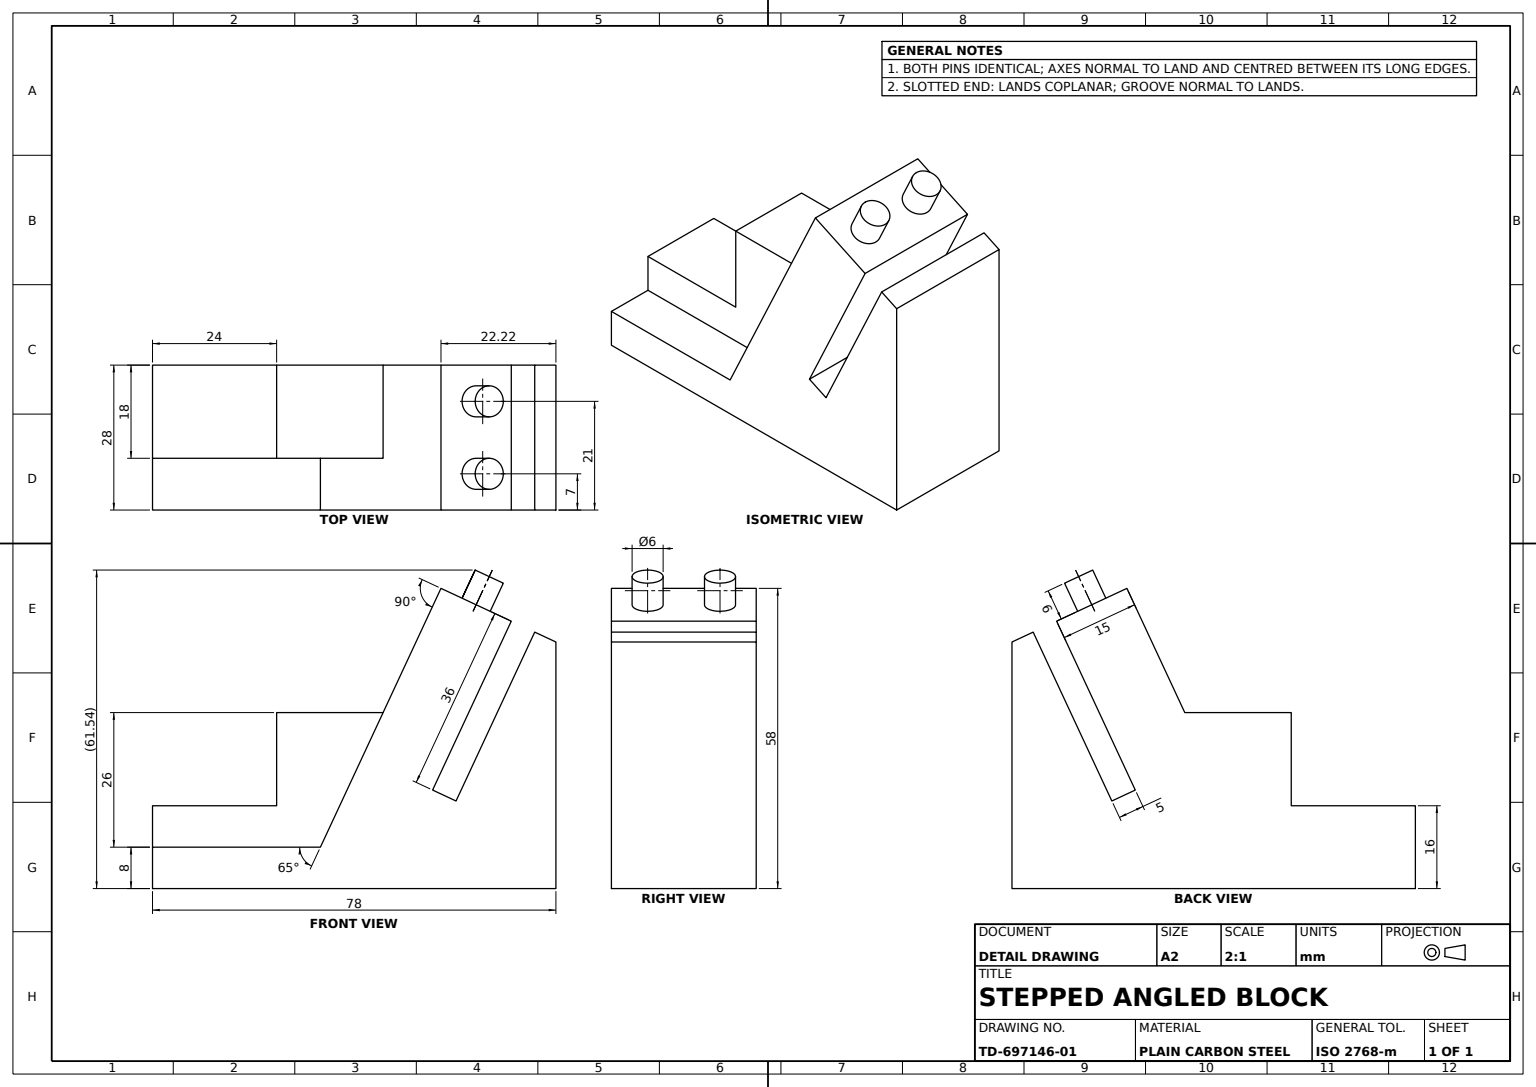
from build123d import *

# Parameters (mm, degrees)
STEPPED_BASE_BLOCK_DEPTH = 28
RISER_BLOCK_16X18_REACH  = 103.153
RISER_BLOCK_SKETCH_W     = 18
RISER_BLOCK_SKETCH_H     = 16
LOCATING_PINS_SKETCH_R   = 3
LOCATING_PINS_X2_DEPTH   = 6
ANGLED_HEAD_SKETCH_W     = 18
ANGLED_HEAD_SKETCH_H     = 18
ANGLED_HEAD_BLOCK_DEPTH  = 26


with BuildPart() as part:
    # Base Profile Sketch → Stepped Base Block (new body)
    with BuildSketch(Plane.XY):
        Polygon((0, 0), (0, 8), (32.461513138, 8), (55.776896046, 58), (69.371512852, 51.660726074), (54.157255429, 19.033645741), (58.688794364, 16.920554432), (73.903051787, 49.547634765), (78, 47.637196438), (78, 0), align=None)
    extrude(amount=STEPPED_BASE_BLOCK_DEPTH)

    # Riser Block 16x18: up to this plane
    riser_block_16x18_end = Plane(origin=(32.461513138, 8, 28), z_dir=(0.9063077870366479, -0.42261826174070377, 0))
    # Riser Block Sketch → Riser Block 16x18 (add, up to the surface)
    with BuildSketch(Plane.ZY, mode=Mode.PRIVATE) as riser_block_16x18_sk1:
        with Locations((9, 8)):
            Rectangle(RISER_BLOCK_SKETCH_W, RISER_BLOCK_SKETCH_H)
    riser_block_16x18_tool1 = split(extrude(riser_block_16x18_sk1.sketch, amount=-RISER_BLOCK_16X18_REACH, mode=Mode.PRIVATE), bisect_by=riser_block_16x18_end, keep=Keep.BOTH, mode=Mode.PRIVATE)
    add(riser_block_16x18_tool1.solids().sort_by_distance((0, 8, 9))[0])

    # Locating Pins Sketch → Locating Pins x2 (add)
    with BuildSketch(Plane(origin=(32.177388031, 69.004631316, 0), x_dir=(0.9063077870366478, -0.42261826174070405, 0), z_dir=(0.4226182617407041, 0.9063077870366479, 0))):
        with Locations((33.539176042, -7)):
            Circle(LOCATING_PINS_SKETCH_R)
        with Locations((33.539176042, -21)):
            Circle(LOCATING_PINS_SKETCH_R)
    extrude(amount=LOCATING_PINS_X2_DEPTH)

    # Angled Head Sketch → Angled Head Block (add)
    with BuildSketch(Plane.ZY.offset(-24)):
        with Locations((9, 25)):
            Rectangle(ANGLED_HEAD_SKETCH_W, ANGLED_HEAD_SKETCH_H)
    extrude(amount=-ANGLED_HEAD_BLOCK_DEPTH)


solid = part.part
